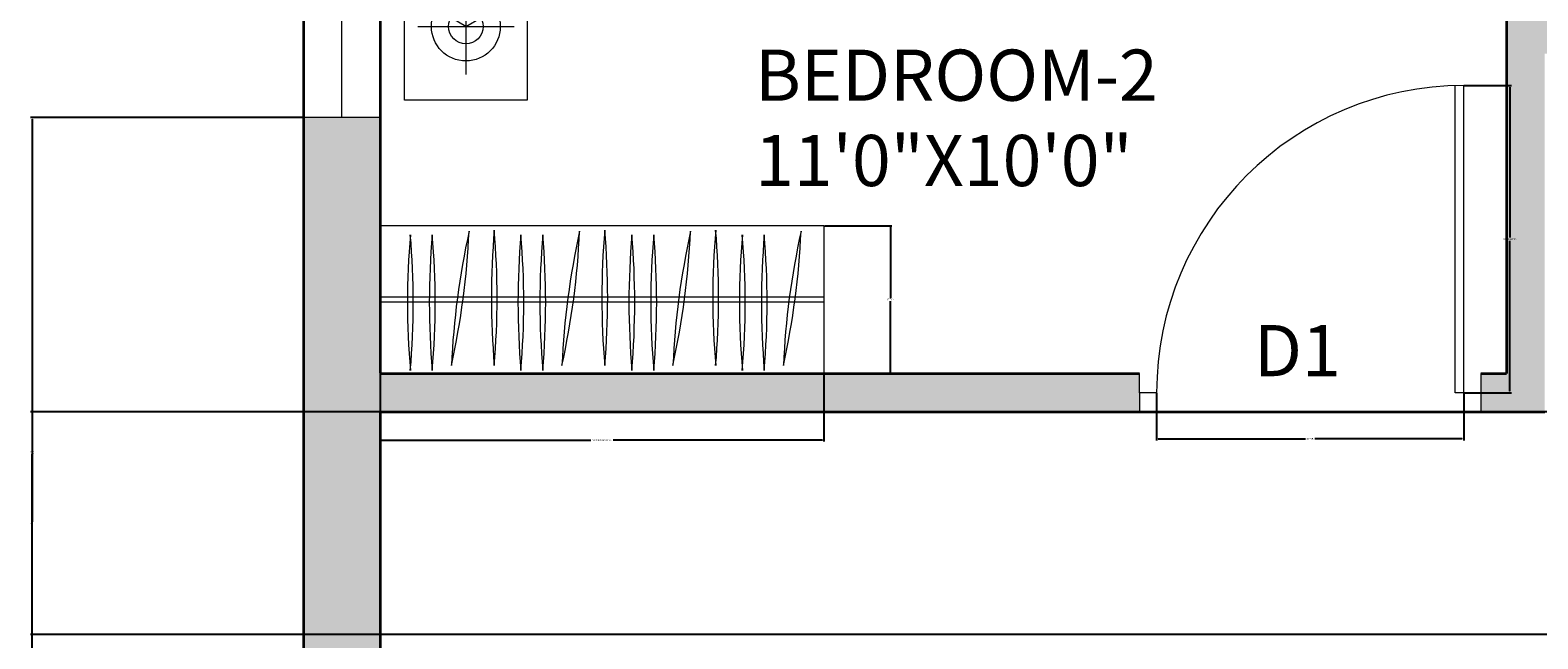
# Model space of a CAD drawing. Units: inches. Extents: x 5 to 421, y -617 to 43.
# Tile 11 of 15: x 5 to 182, y -149 to -78. Entities that reach past the tile are written whole.
import ezdxf

# ---------------------------------------------------------------- set-up
doc = ezdxf.new("R2010")
doc.units = ezdxf.units.IN
doc.header["$MEASUREMENT"] = 0
for name, color, linetype, lineweight in [('A-ANNO-DIMS', 2, 'Continuous', 18), ('A-ANNO-TEXT', 7, 'Continuous', 18), ('A-AREA-IDEN', 7, 'Continuous', 25), ('A-DOOR', 4, 'Continuous', 20), ('A-FLOR-CASE', 8, 'Continuous', 18), ('A-FURN', 8, 'Continuous', 13), ('A-GLAZ', 4, 'Continuous', 18), ('A-WALL', 7, 'Continuous', 35)]:
    doc.layers.add(name, color=color, linetype=linetype, lineweight=lineweight)
doc.layers.add('A-WALL-PATT', color=251, linetype='Continuous', lineweight=13, true_color=0x636466)
doc.styles.get("Standard").update_dxf_attribs({"font": 'arial.ttf'})
doc.dimstyles.get("Standard").update_dxf_attribs({"dimtxt": 0.18, "dimasz": 0.18, "dimexe": 0.18, "dimexo": 0.0625, "dimgap": 0.09, "dimtad": 0, "dimtih": 1, "dimtoh": 1, "dimdec": 0, "dimzin": 0, "dimdsep": 46, "dimlunit": 3, "dimtxsty": 'Standard', "dimcen": 0.09, "dimadec": 0, "dimazin": 0, "dimtfac": 1, "dimtdec": 0, "dimtofl": 0, "dimtmove": 0, "dimatfit": 3, "dimfxl": 1, "dimtolj": 1, "dimtzin": 0, "dimarcsym": 0})

# ---------------------------------------------------------------- blocks, each defined once
blk = doc.blocks.new('WINDOW-W1-60')
for p, q in [((0, 9), (60, 9)), ((0, 0), (0, 9)), ((60, 9), (60, 0)), ((0, 4.5), (60, 4.5)), ((60, 0), (0, 0))]:
    blk.add_line(p, q)
blk = doc.blocks.new('DOOR-SWING-36')
for p, q in [((35, 0), (35, 36)), ((36, 0), (36, 36))]:
    blk.add_line(p, q)
blk.add_arc((36, 0), 36, 90, 180)
blk = doc.blocks.new('WARDROBE-52')
for p, q in [((52, 17.33), (0, 17.33)), ((0, 17.33), (0, 0)), ((52, 17.33), (52, 0)), ((52, 8.96), (0, 8.96)), ((52, 8.38), (0, 8.38)), ((52, 0), (0, 0))]:
    blk.add_line(p, q)
for centre, start, end in [((94.39, 8.32), 175.0028, 184.9972), ((-87.33, 8.32), 355.0028, 4.9972), ((96.95, 8.32), 175.0028, 184.9972), ((-84.76, 8.32), 355.0028, 4.9972), ((-80.71, 20.66), 347.508, 357.5023), ((99.46, -3.04), 167.508, 177.5023), ((104.22, 8.88), 175.0028, 184.9972), ((-77.5, 8.88), 355.0028, 4.9972), ((107.34, 8.32), 175.0028, 184.9972), ((-74.38, 8.32), 355.0028, 4.9972), ((109.91, 8.32), 175.0028, 184.9972), ((-71.81, 8.32), 355.0028, 4.9972), ((-67.75, 20.66), 347.508, 357.5023), ((112.41, -3.04), 167.508, 177.5023), ((117.17, 8.88), 175.0028, 184.9972), ((-64.54, 8.88), 355.0028, 4.9972), ((120.35, 8.32), 175.0028, 184.9972), ((-61.37, 8.32), 355.0028, 4.9972), ((122.91, 8.32), 175.0028, 184.9972), ((-58.8, 8.32), 355.0028, 4.9972), ((125.42, -3.04), 167.508, 177.5023), ((-54.75, 20.66), 347.508, 357.5023), ((130.18, 8.88), 175.0028, 184.9972), ((-51.54, 8.88), 355.0028, 4.9972), ((133.3, 8.32), 175.0028, 184.9972), ((-48.42, 8.32), 355.0028, 4.9972), ((135.87, 8.32), 175.0028, 184.9972), ((-45.85, 8.32), 355.0028, 4.9972), ((138.37, -3.04), 167.508, 177.5023), ((-41.79, 20.66), 347.508, 357.5023)]:
    blk.add_arc(centre, 91.2, start, end)
blk = doc.blocks.new('BEDSIDE-LAMP-DOUBLE')
for p, q in [((5.65, 0), (5.65, 11.29)), ((11.29, 5.65), (0, 5.65))]:
    blk.add_line(p, q)
for points in [[(5.65, 5.65), (3.9, 4.64)], [(5.65, 5.65), (7.39, 4.64)]]:
    blk.add_lwpolyline(points)
for radius in [4.03, 2.02]:
    blk.add_circle((5.65, 5.65), radius)
blk = doc.blocks.new('*D24')
at = {"layer": 'A-ANNO-DIMS', "color": 0, "lineweight": -2, "transparency": 16777216}
for p, q in [((173.48, -84.37), (179, -84.37)), ((178.82, -84.55), (178.82, -102.19)), ((178.82, -120.19), (178.82, -102.55)), ((173.48, -120.37), (179, -120.37))]:
    blk.add_line(p, q, dxfattribs=at)
at = {"layer": 'A-ANNO-DIMS', "color": 0, "transparency": 16777216}
for points in [[(178.79, -84.55), (178.85, -84.55), (178.82, -84.37)], [(178.79, -120.19), (178.85, -120.19), (178.82, -120.37)]]:
    blk.add_solid(points, dxfattribs=at)
at = {"layer": 'Defpoints', "color": 0, "transparency": 16777216}
for p in [(173.42, -84.37), (178.82, -84.37), (173.42, -120.37)]:
    blk.add_point(p, dxfattribs=at)
at = {"layer": 'A-ANNO-DIMS', "color": 0, "transparency": 16777216, "insert": (178.82, -102.37), "char_height": 0.18, "attachment_point": 5}
blk.add_mtext('\\A1;DOOR 36 TYP.', dxfattribs=at)
blk = doc.blocks.new('*D25')
at = {"layer": 'A-ANNO-DIMS', "color": 0, "lineweight": -2, "transparency": 16777216}
for p, q in [((137.42, -120.43), (137.42, -125.95)), ((173.42, -120.43), (173.42, -125.95)), ((137.6, -125.77), (154.89, -125.77)), ((173.24, -125.77), (155.95, -125.77))]:
    blk.add_line(p, q, dxfattribs=at)
at = {"layer": 'A-ANNO-DIMS', "color": 0, "transparency": 16777216}
for points in [[(137.6, -125.74), (137.6, -125.8), (137.42, -125.77)], [(173.24, -125.74), (173.24, -125.8), (173.42, -125.77)]]:
    blk.add_solid(points, dxfattribs=at)
at = {"layer": 'Defpoints', "color": 0, "transparency": 16777216}
for p in [(137.42, -120.37), (173.42, -120.37), (173.42, -125.77)]:
    blk.add_point(p, dxfattribs=at)
at = {"layer": 'A-ANNO-DIMS', "color": 0, "transparency": 16777216, "insert": (155.42, -125.77), "char_height": 0.18, "attachment_point": 5}
blk.add_mtext('\\A1;36 TYP.', dxfattribs=at)
blk = doc.blocks.new('*D40')
at = {"layer": 'A-ANNO-DIMS', "color": 0, "lineweight": -2, "transparency": 16777216}
for p, q in [((46.42, -118.18), (46.42, -126.1)), ((98.42, -118.18), (98.42, -126.1)), ((46.6, -125.92), (71.11, -125.92)), ((98.24, -125.92), (73.73, -125.92))]:
    blk.add_line(p, q, dxfattribs=at)
at = {"layer": 'A-ANNO-DIMS', "color": 0, "transparency": 16777216}
for points in [[(46.6, -125.89), (46.6, -125.95), (46.42, -125.92)], [(98.24, -125.89), (98.24, -125.95), (98.42, -125.92)]]:
    blk.add_solid(points, dxfattribs=at)
at = {"layer": 'Defpoints', "color": 0, "transparency": 16777216}
for p in [(46.42, -118.12), (98.42, -118.12), (98.42, -125.92)]:
    blk.add_point(p, dxfattribs=at)
at = {"layer": 'A-ANNO-DIMS', "color": 0, "transparency": 16777216, "insert": (72.42, -125.92), "char_height": 0.18, "attachment_point": 5}
blk.add_mtext('\\A1;WARDROBE 52 TYP.', dxfattribs=at)
blk = doc.blocks.new('*D41')
at = {"layer": 'A-ANNO-DIMS', "color": 0, "lineweight": -2, "transparency": 16777216}
for p, q in [((98.48, -100.79), (106.4, -100.79)), ((106.22, -100.97), (106.22, -109.27)), ((106.22, -117.94), (106.22, -109.63)), ((98.48, -118.12), (106.4, -118.12))]:
    blk.add_line(p, q, dxfattribs=at)
at = {"layer": 'A-ANNO-DIMS', "color": 0, "transparency": 16777216}
for points in [[(106.19, -100.97), (106.25, -100.97), (106.22, -100.79)], [(106.19, -117.94), (106.25, -117.94), (106.22, -118.12)]]:
    blk.add_solid(points, dxfattribs=at)
at = {"layer": 'Defpoints', "color": 0, "transparency": 16777216}
for p in [(98.42, -100.79), (106.22, -100.79), (98.42, -118.12)]:
    blk.add_point(p, dxfattribs=at)
at = {"layer": 'A-ANNO-DIMS', "color": 0, "transparency": 16777216, "insert": (106.22, -109.45), "char_height": 0.18, "attachment_point": 5}
blk.add_mtext('\\A1;17 TYP.', dxfattribs=at)
blk = doc.blocks.new('*D54')
at = {"layer": 'A-ANNO-DIMS', "color": 0, "lineweight": -2, "transparency": 16777216}
for p, q in [((37.42, 10.94), (37.42, 42.86)), ((37.6, 42.68), (212.65, 42.68)), ((388.24, 42.68), (213.19, 42.68)), ((388.42, -118.06), (388.42, 42.86))]:
    blk.add_line(p, q, dxfattribs=at)
at = {"layer": 'A-ANNO-DIMS', "color": 0, "transparency": 16777216}
for points in [[(37.6, 42.71), (37.6, 42.65), (37.42, 42.68)], [(388.24, 42.71), (388.24, 42.65), (388.42, 42.68)]]:
    blk.add_solid(points, dxfattribs=at)
at = {"layer": 'Defpoints', "color": 0, "transparency": 16777216}
for p in [(37.42, 42.68), (37.42, 10.88), (388.42, -118.12)]:
    blk.add_point(p, dxfattribs=at)
at = {"layer": 'A-ANNO-DIMS', "color": 0, "transparency": 16777216, "insert": (212.92, 42.68), "char_height": 0.18, "attachment_point": 5}
blk.add_mtext('\\A1;351', dxfattribs=at)
blk = doc.blocks.new('*D55')
at = {"layer": 'A-ANNO-DIMS', "color": 0, "lineweight": -2, "transparency": 16777216}
for p, q in [((370.48, 10.88), (420.4, 10.88)), ((420.22, 10.7), (420.22, -286.69)), ((420.22, -584.44), (420.22, -287.05)), ((169.48, -584.62), (420.4, -584.62))]:
    blk.add_line(p, q, dxfattribs=at)
at = {"layer": 'A-ANNO-DIMS', "color": 0, "transparency": 16777216}
for points in [[(420.19, 10.7), (420.25, 10.7), (420.22, 10.88)], [(420.19, -584.44), (420.25, -584.44), (420.22, -584.62)]]:
    blk.add_solid(points, dxfattribs=at)
at = {"layer": 'Defpoints', "color": 0, "transparency": 16777216}
for p in [(370.42, 10.88), (169.42, -584.62), (420.22, -584.62)]:
    blk.add_point(p, dxfattribs=at)
at = {"layer": 'A-ANNO-DIMS', "color": 0, "transparency": 16777216, "insert": (420.22, -286.87), "char_height": 0.18, "attachment_point": 5}
blk.add_mtext('\\A1;595.5', dxfattribs=at)
blk = doc.blocks.new('*D61')
at = {"layer": 'A-ANNO-DIMS', "color": 0, "lineweight": -2, "transparency": 16777216}
for p, q in [((37.36, -88.12), (5.44, -88.12)), ((5.62, -88.3), (5.62, -127.18)), ((5.62, -166.43), (5.62, -127.55)), ((37.36, -166.61), (5.44, -166.61))]:
    blk.add_line(p, q, dxfattribs=at)
at = {"layer": 'A-ANNO-DIMS', "color": 0, "transparency": 16777216}
for points in [[(5.59, -88.3), (5.65, -88.3), (5.62, -88.12)], [(5.59, -166.43), (5.65, -166.43), (5.62, -166.61)]]:
    blk.add_solid(points, dxfattribs=at)
at = {"layer": 'Defpoints', "color": 0, "transparency": 16777216}
for p in [(37.42, -88.12), (5.62, -166.61), (37.42, -166.61)]:
    blk.add_point(p, dxfattribs=at)
at = {"layer": 'A-ANNO-DIMS', "color": 0, "transparency": 16777216, "insert": (5.62, -127.37), "char_height": 0.18, "attachment_point": 5}
blk.add_mtext('\\A1;78.5', dxfattribs=at)
blk = doc.blocks.new('*D68')
at = {"layer": 'A-ANNO-DIMS', "color": 0, "lineweight": -2, "transparency": 16777216}
for p, q in [((224.86, -122.62), (5.44, -122.62)), ((5.62, -122.8), (5.62, -135.49)), ((5.62, -148.54), (5.62, -135.85)), ((224.86, -148.72), (5.44, -148.72))]:
    blk.add_line(p, q, dxfattribs=at)
at = {"layer": 'A-ANNO-DIMS', "color": 0, "transparency": 16777216}
for points in [[(5.59, -122.8), (5.65, -122.8), (5.62, -122.62)], [(5.59, -148.54), (5.65, -148.54), (5.62, -148.72)]]:
    blk.add_solid(points, dxfattribs=at)
at = {"layer": 'Defpoints', "color": 0, "transparency": 16777216}
for p in [(224.92, -122.62), (5.62, -148.72), (224.92, -148.72)]:
    blk.add_point(p, dxfattribs=at)
at = {"layer": 'A-ANNO-DIMS', "color": 0, "transparency": 16777216, "insert": (5.62, -135.67), "char_height": 0.18, "attachment_point": 5}
blk.add_mtext('\\A1;26.1', dxfattribs=at)

msp = doc.modelspace()

# ---------------------------------------------------------------- hatches: boundary and pattern name
at = {"layer": 'A-WALL-PATT'}
h = msp.add_hatch(color=256, dxfattribs=at)
h.dxf.hatch_style = 1
h.paths.add_polyline_path([(46.4196, -88.1188), (37.4196, -88.1188), (37.4196, -166.6119), (46.4196, -166.6119), (46.4196, -122.6188), (135.4196, -122.6188), (135.4196, -120.3688), (135.4196, -118.1188), (46.4196, -118.1188)])
h.paths.add_polyline_path([(82.4196, 10.8812), (37.4196, 10.8812), (37.4196, -28.1188), (46.4196, -28.1188), (46.4196, 1.8812), (82.4196, 1.8812)])
h.paths.add_polyline_path([(215.5968, 10.8812), (142.4196, 10.8812), (142.4196, 1.8812), (178.4196, 1.8812), (178.4196, -118.1188), (175.4196, -118.1188), (175.4196, -122.6188), (182.9196, -122.6188), (182.9196, -80.6188), (211.9196, -80.6188), (211.9196, -78.3688), (211.9196, -76.1188), (182.9196, -76.1188), (182.9196, 1.8812), (215.5968, 1.8812)])
h.paths.add_polyline_path([(274.4196, 10.8812), (239.5968, 10.8812), (239.5968, 1.8812), (242.9196, 1.8812), (242.9196, -76.1188), (239.9196, -76.1188), (239.9196, -80.6188), (242.9196, -80.6188), (242.9196, -83.6188), (247.4196, -83.6188), (247.4196, 1.8812), (274.4196, 1.8812)])
h.paths.add_polyline_path([(370.4196, 10.8812), (334.4196, 10.8812), (334.4196, 1.8812), (361.4196, 1.8812), (361.4196, -28.1188), (370.4196, -28.1188)])
h.paths.add_polyline_path([(370.4196, -88.1188), (361.4196, -88.1188), (361.4196, -118.1188), (247.4196, -118.1188), (247.4196, -115.1188), (242.9196, -115.1188), (242.9196, -118.1188), (220.4196, -118.1188), (220.4196, -158.6188), (224.9196, -158.6188), (224.9196, -122.6188), (326.9196, -122.6188), (326.9196, -170.7662), (331.4196, -170.7662), (331.4196, -122.6188), (370.4196, -122.6188)])
h.paths.add_polyline_path([(388.4196, -122.6188), (388.4196, -118.1188), (379.4196, -118.1188), (379.4196, -122.6188), (379.4196, -154.8688), (388.4196, -154.8688)])
h.paths.add_polyline_path([(388.4196, -214.8688), (379.4196, -214.8688), (379.4196, -247.1188), (388.4196, -247.1188)])
h.paths.add_polyline_path([(371.0265, -242.6188), (331.4196, -242.6188), (331.4196, -239.6188), (326.9196, -239.6188), (326.9196, -242.6188), (224.9196, -242.6188), (224.9196, -206.6188), (220.4196, -206.6188), (220.4196, -343.6188), (224.9196, -343.6188), (229.4196, -343.6188), (229.4196, -247.1188), (261.5265, -247.1188), (261.5265, -276.1188), (263.7765, -276.1188), (266.0265, -276.1188), (266.0265, -247.1188), (362.0265, -247.1188), (362.0265, -265.1188), (371.0265, -265.1188), (371.0265, -247.1188)])
h.paths.add_polyline_path([(371.0265, -289.1188), (362.0265, -289.1188), (362.0265, -307.1188), (266.0265, -307.1188), (266.0265, -304.1188), (261.5265, -304.1188), (261.5265, -307.1188), (261.5265, -311.6188), (362.0265, -311.6188), (362.0265, -353.6188), (371.0265, -353.6188)])
h.paths.add_polyline_path([(371.0265, -413.6188), (362.0265, -413.6188), (362.0265, -455.6188), (325.7231, -455.6188), (325.7231, -464.6188), (361.4196, -464.6188), (371.0265, -464.6188)])
h.paths.add_polyline_path([(265.7231, -455.6188), (229.4196, -455.6188), (229.4196, -383.6188), (220.4196, -383.6188), (220.4196, -386.6188), (207.4649, -386.6188), (207.4649, -395.6188), (220.4196, -395.6188), (220.4196, -455.6188), (216.0568, -455.6188), (216.0568, -464.6188), (265.7231, -464.6188)])
h.paths.add_polyline_path([(169.4196, -386.6188), (137.9196, -386.6188), (137.9196, -395.6188), (160.4196, -395.6188), (160.4196, -424.2032), (169.4196, -424.2032)])
h.paths.add_polyline_path([(169.4196, -453.7423), (160.4196, -453.7423), (160.4196, -464.6188), (169.4196, -464.6188)])
h.paths.add_polyline_path([(46.4196, -575.6188), (37.4196, -575.6188), (37.4196, -584.6188), (46.4196, -584.6188)])
h.paths.add_polyline_path([(169.4196, -575.6188), (160.4196, -575.6188), (160.4196, -579.5504), (160.4196, -584.6188), (169.4196, -584.6188)])
h.paths.add_polyline_path([(46.4196, -226.6119), (37.4196, -226.6119), (37.4196, -292.8008), (46.4196, -292.8008)])
h.paths.add_polyline_path([(46.4196, -352.8008), (37.4196, -352.8008), (37.4196, -395.6188), (77.9196, -395.6188), (77.9196, -386.6188), (46.4196, -386.6188)])

# ---------------------------------------------------------------- linework, layer by layer
at = {"layer": 'A-DOOR'}
for p, q in [((135.4196, -120.3688), (135.4196, -118.1188)), ((175.4196, -118.1188), (175.4196, -122.6188)), ((137.4196, -120.3688), (135.4196, -120.3688)), ((135.4196, -120.3688), (135.4196, -122.6188)), ((175.4196, -120.3688), (172.4196, -120.3688))]:
    msp.add_line(p, q, dxfattribs=at)
at = {"layer": 'A-FURN'}
msp.add_line((49.2533, -86.083), (49.2533, 0.3477), dxfattribs=at)
msp.add_lwpolyline([(63.6585, -68.7969), (63.6585, -86.083), (49.2533, -86.083)], dxfattribs=at)
at = {"layer": 'A-WALL'}
for p, q in [((37.4196, 10.8812), (37.4196, -584.6188)), ((46.4196, 1.8812), (46.4196, -118.1188)), ((178.4196, 1.8812), (178.4196, -118.1188)), ((46.4196, -118.1188), (135.4196, -118.1188)), ((175.4196, -118.1188), (178.4196, -118.1188)), ((46.4196, -122.6188), (182.9196, -122.6188)), ((46.4196, -122.6188), (46.4196, -386.6188))]:
    msp.add_line(p, q, dxfattribs=at)

# ---------------------------------------------------------------- block references
at = {"layer": 'A-DOOR'}
msp.add_blockref('DOOR-SWING-36', (137.4196, -120.3688), dxfattribs=at)
at = {"layer": 'A-FLOR-CASE'}
msp.add_blockref('WARDROBE-52', (46.4196, -118.1188), dxfattribs=at)
at = {"layer": 'A-FURN', "rotation": 180}
msp.add_blockref('BEDSIDE-LAMP-DOUBLE', (62.1027, -71.7932), dxfattribs=at)
at = {"layer": 'A-GLAZ', "rotation": 90.00000000000003}
msp.add_blockref('WINDOW-W1-60', (46.4196, -88.1188), dxfattribs=at)

# ---------------------------------------------------------------- texts
at = {"layer": 'A-ANNO-TEXT', "insert": (148.8328, -112.4285), "char_height": 6, "attachment_point": 1}
msp.add_mtext('D1', dxfattribs=at)
at = {"layer": 'A-AREA-IDEN', "insert": (90.3506, -80.1493), "char_height": 6, "attachment_point": 1}
msp.add_mtext('BEDROOM-2\\P11\'0"X10\'0"', dxfattribs=at)

# ---------------------------------------------------------------- dimensions: what is measured, and where the dimension line sits
at = {"layer": 'A-ANNO-DIMS'}
dim = msp.add_linear_dim(base=(37.4196, 42.6812), p1=(388.4196, -118.1188), p2=(37.4196, 10.8812), dimstyle='Standard', override={"dimdec": 0, "dimlfac": 1, "dimrnd": 0, "dimzin": 0, "dimdsep": 46, "dimlunit": 2}, dxfattribs=at)
dim.commit()
dim.dimension.update_dxf_attribs({"geometry": '*D54', "text_midpoint": (212.9196, 42.6812)})
for base, p1, p2, picture, middle in [((420.2196, -584.6188), (370.4196, 10.8812), (169.4196, -584.6188), '*D55', (420.2196, -286.8688)), ((5.6196, -166.6119), (37.4196, -88.1188), (37.4196, -166.6119), '*D61', (5.6196, -127.3654)), ((5.6196, -148.7194), (224.9196, -122.6188), (224.9196, -148.7194), '*D68', (5.6196, -135.6691))]:
    dim = msp.add_linear_dim(base=base, p1=p1, p2=p2, angle=90, dimstyle='Standard', override={"dimdec": 1, "dimlfac": 1, "dimrnd": 0, "dimzin": 0, "dimdsep": 46, "dimlunit": 2}, dxfattribs=at)
    dim.commit()
    dim.dimension.update_dxf_attribs({"geometry": picture, "text_midpoint": middle})
for base, p1, p2, text, picture, middle in [((178.8196, -84.3688), (173.4196, -120.3688), (173.4196, -84.3688), 'DOOR <> TYP.', '*D24', (178.8196, -102.3688)), ((106.2206, -100.7852), (98.4205, -118.1188), (98.4205, -100.7852), '<> TYP.', '*D41', (106.2206, -109.452))]:
    dim = msp.add_linear_dim(base=base, p1=p1, p2=p2, angle=90, text=text, dimstyle='Standard', override={"dimdec": 0, "dimlfac": 1, "dimrnd": 0, "dimzin": 0, "dimdsep": 46, "dimlunit": 2}, dxfattribs=at)
    dim.commit()
    dim.dimension.update_dxf_attribs({"geometry": picture, "text_midpoint": middle})
for base, p1, p2, text, picture, middle in [((98.4205, -125.919), (46.4196, -118.1188), (98.4205, -118.1188), 'WARDROBE <> TYP.', '*D40', (72.42, -125.919)), ((173.4196, -125.7688), (137.4196, -120.3688), (173.4196, -120.3688), '<> TYP.', '*D25', (155.4196, -125.7688))]:
    dim = msp.add_linear_dim(base=base, p1=p1, p2=p2, text=text, dimstyle='Standard', override={"dimdec": 0, "dimlfac": 1, "dimrnd": 0, "dimzin": 0, "dimdsep": 46, "dimlunit": 2}, dxfattribs=at)
    dim.commit()
    dim.dimension.update_dxf_attribs({"geometry": picture, "text_midpoint": middle})

doc.saveas('drawing.dxf')
